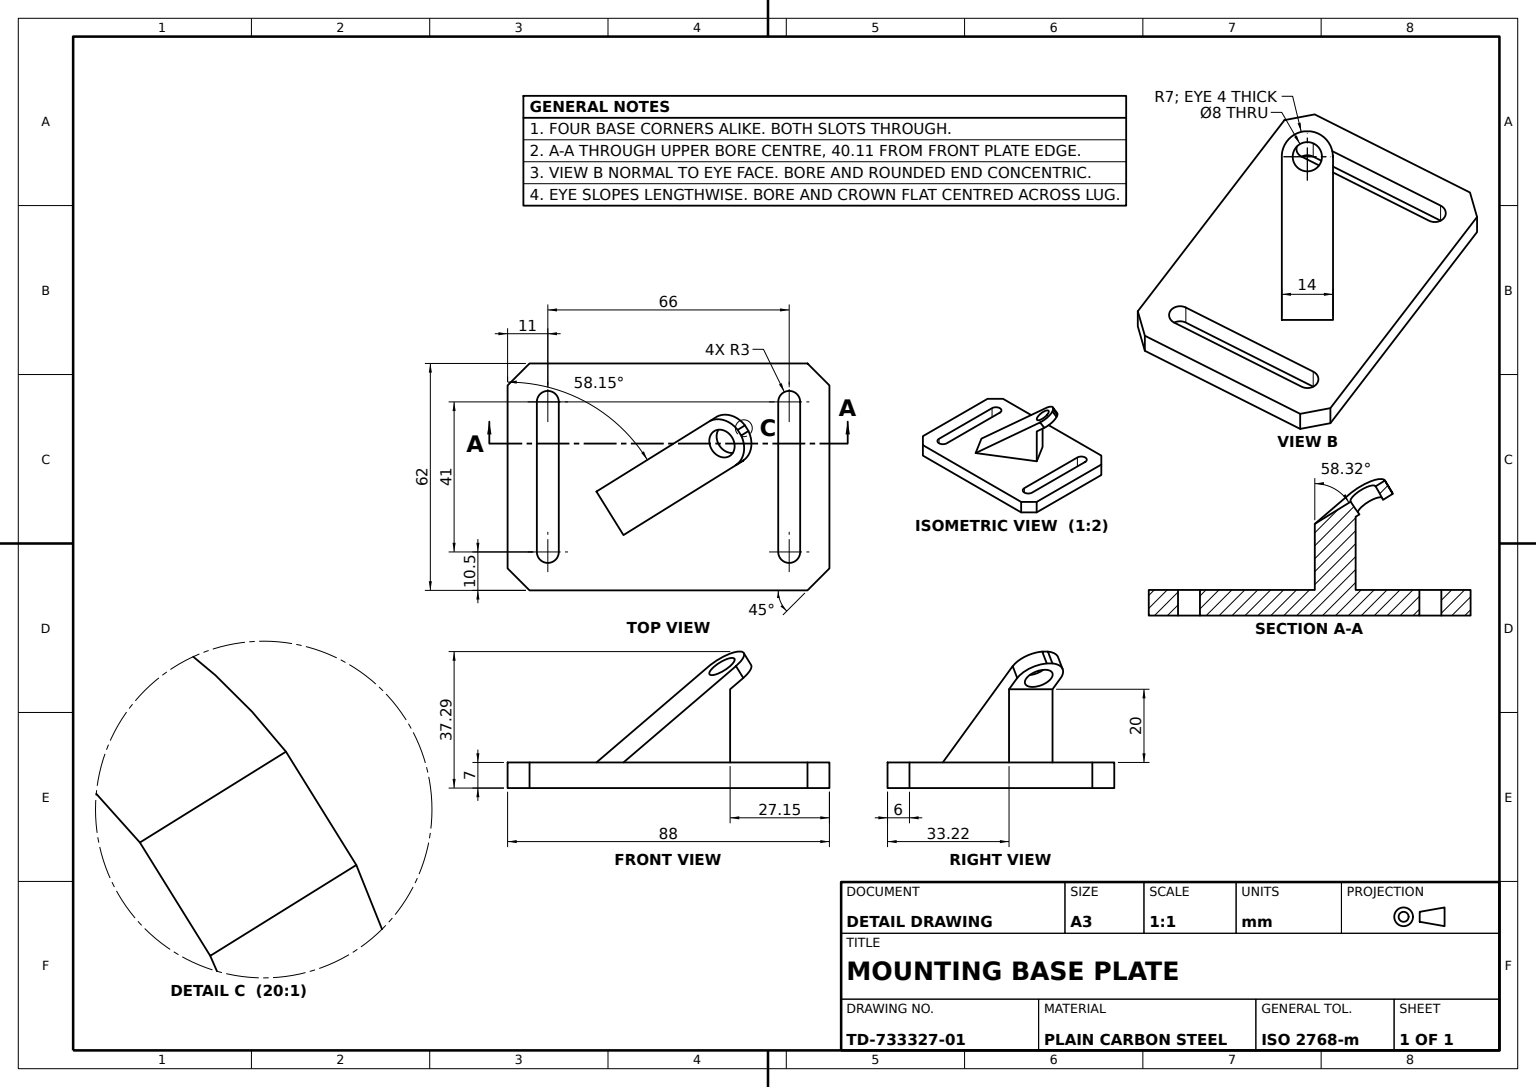
from build123d import *

# Parameters (mm, degrees)
BASE_PLATE_PROFILE_W        = 88
BASE_PLATE_PROFILE_H        = 62
BASE_PLATE_88X62X7_DEPTH    = 7
PLATE_EDGE_CHAMFER_6MM_SIZE = 6
LIFTING_LUG_DEPTH           = 87
LUG_TAPER_CUT_DEPTH         = 87
LUG_TRIM_CUT_DEPTH          = 7
LUG_EYE_HOLE_PROFILE_R      = 4
LUG_EYE_HOLE_DEPTH          = 17


with BuildPart() as part:
    # Base Plate Profile → Base Plate 88x62x7 (new body)
    with BuildSketch(Plane(origin=(0, 0, 0), x_dir=(1, 0, 0), z_dir=(0, 1, 0))):
        Rectangle(BASE_PLATE_PROFILE_W, BASE_PLATE_PROFILE_H)
        with BuildLine():
            Line((-30, 20.5), (-30, -20.5))
            ThreePointArc((-30, -20.5), (-33, -23.5), (-36, -20.5))
            Line((-36, -20.5), (-36, 20.5))
            ThreePointArc((-36, 20.5), (-33, 23.5), (-30, 20.5))
        make_face(mode=Mode.SUBTRACT)
        with BuildLine():
            Line((36, 20.5), (36, -20.5))
            ThreePointArc((36, -20.5), (33, -23.5), (30, -20.5))
            Line((30, -20.5), (30, 20.5))
            ThreePointArc((30, 20.5), (33, 23.5), (36, 20.5))
        make_face(mode=Mode.SUBTRACT)
    extrude(amount=BASE_PLATE_88X62X7_DEPTH)

    # Plate Edge Chamfer 6mm
    plate_edge_chamfer_6mm_edges = [part.edges().sort_by_distance(p)[0] for p in [
        (44, 3.5, 31),
        (-44, 3.5, 31),
        (-44, 3.5, -31),
        (44, 3.5, -31),
    ]]
    chamfer(plate_edge_chamfer_6mm_edges, length=PLATE_EDGE_CHAMFER_6MM_SIZE)

    # Lug Profile → Lifting Lug (add)
    with BuildSketch(Plane(origin=(0, 7, 0), x_dir=(1, 0, 0), z_dir=(0, 1, 0))):
        Polygon((-19.704957389, -4.000247215), (-12.317392569, -15.892424729), (49.796954416, 22.693760519), (42.409389597, 34.585938034), align=None)
    extrude(amount=LIFTING_LUG_DEPTH)

    # Lug Taper Cut Profile → Lug Taper Cut (cut)
    with BuildSketch(Plane(origin=(3.69378241, 0, 5.946088757), x_dir=(0.849441251034907, 0, -0.527683201400473), z_dir=(0.527683201400473, 0, 0.8494412510349071))):
        Polygon((-18.849066913, 7), (22.840840887, 37.289491005), (25.191981896, 34.053423028), (15.483777963, 27), (15.483777963, 7), (61.160327949, 7), (67.88344363, 13.003001153), (104.454353656, 45.656792269), (102.884273853, 93.151706309), (-3.096112848, 106.69364461), (-91.21684179, 88.04894695), align=None)
    extrude(amount=-LUG_TAPER_CUT_DEPTH, mode=Mode.SUBTRACT)

    # Lug Trim Profile → Lug Trim Cut (cut)
    with BuildSketch(Plane(origin=(-8.359258135, 13.544823437, 5.192872478), x_dir=(0.8664354877824213, 0.46620126275894425, 0.17873423878262307), z_dir=(-0.4992890400471833, 0.8090169943749503, 0.31016440366567466))):
        with BuildLine():
            Line((21.785997787, 25.554185682), (25.412738519, 37.418943579))
            Line((25.412738519, 37.418943579), (44.862853062, 15.660355845))
            Line((44.862853062, 15.660355845), (35.13779579, 16.937383568))
            Line((35.13779579, 16.937383568), (30.824168068, 14.877305743))
            ThreePointArc((30.824168068, 14.877305743), (31.862256086, 24.919992419), (21.785997787, 25.554185682))
        make_face()
    extrude(amount=-LUG_TRIM_CUT_DEPTH, mode=Mode.SUBTRACT)

    # Lug Eye Hole Profile → Lug Eye Hole (cut)
    with BuildSketch(Plane(origin=(-8.359258135, 13.544823437, 5.192872478), x_dir=(0.8664354877824213, 0.46620126275894425, 0.17873423878262307), z_dir=(-0.4992890400471833, 0.8090169943749503, 0.31016440366567466))):
        with Locations(Location((26.519511391, 20.397263251, 0), (0, 0, 190.836448225))):
            Circle(LUG_EYE_HOLE_PROFILE_R)
    extrude(amount=-LUG_EYE_HOLE_DEPTH, mode=Mode.SUBTRACT)


solid = part.part
